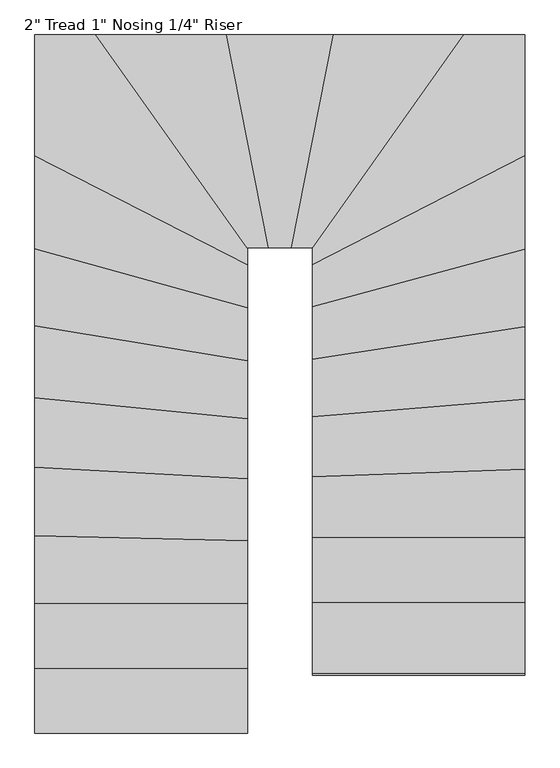
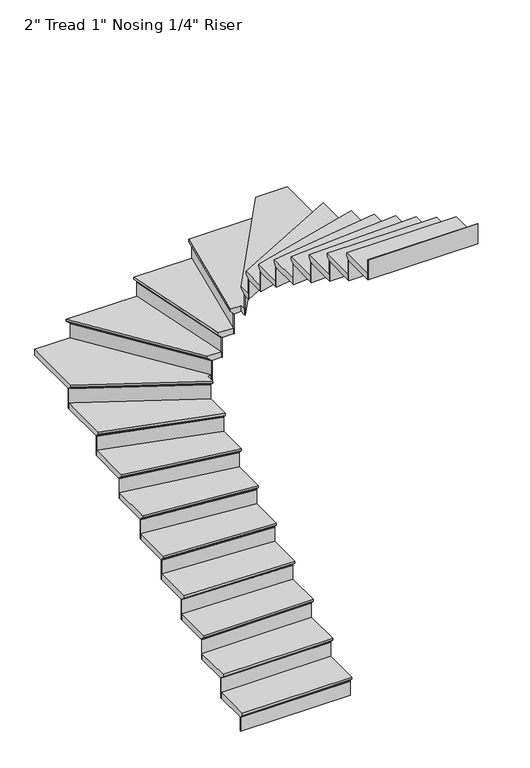
"""IFC4 building model written with IfcOpenShell, lengths in millimetres: stair flight geometry."""

from ifc_helpers import new_model, si_unit, origin, place, context, project, spatial, faceted_brep, source, transform, mapped, element, save


def stair_flight_b5c60846(model_context):
    return source(origin(), model_context, "Body", "Brep", [
        faceted_brep([(-4558.1931367, 3267.4797066, 155.1214286), (-4558.1931367, 3267.4797066, 174.1714286), (-5472.5931367, 3267.4797066, 174.1714286), (-5472.5931367, 3267.4797066, 155.1214286), (-4558.1931367, 3292.8797066, 129.7214286), (-5472.5931367, 3292.8797066, 129.7214286), (-4558.1931367, 3572.2797066, 174.1714286), (-5472.5931367, 3572.2797066, 174.1714286), (-5472.5931367, 3292.8797066, 123.3714286), (-5472.5931367, 3572.2797066, 123.3714286), (-4558.1931367, 3572.2797066, 123.3714286), (-4558.1931367, 3292.8797066, 123.3714286)], [[[0, 1, 2, 3]], [[4, 0, 3, 5]], [[2, 1, 6, 7]], [[8, 9, 10, 11]], [[2, 7, 9, 8, 5, 3]], [[8, 11, 4, 5]], [[6, 1, 0, 4, 11, 10]], [[7, 6, 10, 9]]]),
        faceted_brep([(-4558.1931367, 3292.8797066, 123.3714286), (-4558.1931367, 3292.8797066, 0.0), (-4558.1931367, 3299.2297066, 0.0), (-4558.1931367, 3299.2297066, 123.3714286), (-5472.5931367, 3292.8797066, 123.3714286), (-5472.5931367, 3299.2297066, 123.3714286), (-5472.5931367, 3299.2297066, 0.0), (-5472.5931367, 3292.8797066, 0.0)], [[[0, 1, 2, 3]], [[4, 5, 6, 7]], [[1, 0, 4, 7]], [[2, 1, 7, 6]], [[3, 2, 6, 5]], [[0, 3, 5, 4]]]),
        faceted_brep([(-4558.1931367, 3572.2797066, 297.5428571), (-4558.1931367, 3572.2797066, 123.3714286), (-4558.1931367, 3578.6297066, 123.3714286), (-4558.1931367, 3578.6297066, 297.5428571), (-5472.5931367, 3572.2797066, 297.5428571), (-5472.5931367, 3578.6297066, 297.5428571), (-5472.5931367, 3578.6297066, 123.3714286), (-5472.5931367, 3572.2797066, 123.3714286)], [[[0, 1, 2, 3]], [[4, 5, 6, 7]], [[1, 0, 4, 7]], [[2, 1, 7, 6]], [[3, 2, 6, 5]], [[0, 3, 5, 4]]]),
        faceted_brep([(-5472.5931367, 3546.8797066, 348.3428571), (-4558.1931367, 3546.8797066, 348.3428571), (-4558.1931367, 3851.6797066, 348.3428571), (-5472.5931367, 3851.6797066, 348.3428571), (-5472.5931367, 3572.2797066, 297.5428571), (-5472.5931367, 3851.6797066, 297.5428571), (-4558.1931367, 3851.6797066, 297.5428571), (-4558.1931367, 3572.2797066, 297.5428571), (-5472.5931367, 3572.2797066, 303.8928571), (-5472.5931367, 3546.8797066, 329.2928571), (-4558.1931367, 3572.2797066, 303.8928571), (-4558.1931367, 3546.8797066, 329.2928571)], [[[0, 1, 2, 3]], [[4, 5, 6, 7]], [[0, 3, 5, 4, 8, 9]], [[4, 7, 10, 8]], [[2, 1, 11, 10, 7, 6]], [[3, 2, 6, 5]], [[11, 1, 0, 9]], [[10, 11, 9, 8]]]),
        faceted_brep([(-4558.1931367, 3851.6797066, 471.7142857), (-4558.1931367, 3851.6797066, 297.5428571), (-4558.1931367, 3858.0297066, 297.5428571), (-4558.1931367, 3858.0297066, 471.7142857), (-5472.5931367, 3851.6797066, 471.7142857), (-5472.5931367, 3858.0297066, 471.7142857), (-5472.5931367, 3858.0297066, 297.5428571), (-5472.5931367, 3851.6797066, 297.5428571)], [[[0, 1, 2, 3]], [[4, 5, 6, 7]], [[1, 0, 4, 7]], [[2, 1, 7, 6]], [[3, 2, 6, 5]], [[0, 3, 5, 4]]]),
        faceted_brep([(-5472.5931367, 3826.2797066, 522.5142857), (-4558.1931367, 3826.2797066, 522.5142857), (-4558.1931367, 4120.4786565, 522.5142857), (-5472.5931367, 4141.6944283, 522.5142857), (-5472.5931367, 3851.6797066, 471.7142857), (-5472.5931367, 4141.6944283, 471.7142857), (-4558.1931367, 4120.4786565, 471.7142857), (-4558.1931367, 3851.6797066, 471.7142857), (-5472.5931367, 3851.6797066, 478.0642857), (-5472.5931367, 3826.2797066, 503.4642857), (-4558.1931367, 3851.6797066, 478.0642857), (-4558.1931367, 3826.2797066, 503.4642857)], [[[0, 1, 2, 3]], [[4, 5, 6, 7]], [[0, 3, 5, 4, 8, 9]], [[4, 7, 10, 8]], [[2, 1, 11, 10, 7, 6]], [[3, 2, 6, 5]], [[11, 1, 0, 9]], [[10, 11, 9, 8]]]),
        faceted_brep([(-4558.1931367, 4120.4786565, 645.8857143), (-4558.1931367, 4120.4786565, 471.7142857), (-4558.1931367, 4126.8303655, 471.7142857), (-4558.1931367, 4126.8303655, 645.8857143), (-5472.5931367, 4141.6944283, 645.8857143), (-5472.5931367, 4148.0461372, 645.8857143), (-5472.5931367, 4148.0461372, 471.7142857), (-5472.5931367, 4141.6944283, 471.7142857)], [[[0, 1, 2, 3]], [[4, 5, 6, 7]], [[1, 0, 4, 7]], [[2, 1, 7, 6]], [[3, 2, 6, 5]], [[0, 3, 5, 4]]]),
        faceted_brep([(-5472.5931367, 4116.2875924, 696.6857143), (-4558.1931367, 4095.0718207, 696.6857143), (-4558.1931367, 4385.6939265, 696.6857143), (-5472.5931367, 4435.3403065, 696.6857143), (-5472.5931367, 4141.6944283, 645.8857143), (-5472.5931367, 4435.3403065, 645.8857143), (-4558.1931367, 4385.6939265, 645.8857143), (-4558.1931367, 4120.4786565, 645.8857143), (-5472.5931367, 4141.6944283, 652.2357143), (-5472.5931367, 4116.2875924, 677.6357143), (-4558.1931367, 4120.4786565, 652.2357143), (-4558.1931367, 4095.0718207, 677.6357143)], [[[0, 1, 2, 3]], [[4, 5, 6, 7]], [[0, 3, 5, 4, 8, 9]], [[4, 7, 10, 8]], [[2, 1, 11, 10, 7, 6]], [[3, 2, 6, 5]], [[11, 1, 0, 9]], [[10, 11, 9, 8]]]),
        faceted_brep([(-4558.1931367, 4385.6939265, 820.0571429), (-4558.1931367, 4385.6939265, 645.8857143), (-4558.1931367, 4392.053279, 645.8857143), (-4558.1931367, 4392.053279, 820.0571429), (-5472.5931367, 4435.3403065, 820.0571429), (-5472.5931367, 4441.699659, 820.0571429), (-5472.5931367, 4441.699659, 645.8857143), (-5472.5931367, 4435.3403065, 645.8857143)], [[[0, 1, 2, 3]], [[4, 5, 6, 7]], [[1, 0, 4, 7]], [[2, 1, 7, 6]], [[3, 2, 6, 5]], [[0, 3, 5, 4]]]),
        faceted_brep([(-5472.5931367, 4409.9028966, 870.8571429), (-4558.1931367, 4360.2565166, 870.8571429), (-4558.1931367, 4645.138633, 870.8571429), (-5472.5931367, 4734.864762, 870.8571429), (-5472.5931367, 4435.3403065, 820.0571429), (-5472.5931367, 4734.864762, 820.0571429), (-4558.1931367, 4645.138633, 820.0571429), (-4558.1931367, 4385.6939265, 820.0571429), (-5472.5931367, 4435.3403065, 826.4071429), (-5472.5931367, 4409.9028966, 851.8071429), (-4558.1931367, 4385.6939265, 826.4071429), (-4558.1931367, 4360.2565166, 851.8071429)], [[[0, 1, 2, 3]], [[4, 5, 6, 7]], [[0, 3, 5, 4, 8, 9]], [[4, 7, 10, 8]], [[2, 1, 11, 10, 7, 6]], [[3, 2, 6, 5]], [[11, 1, 0, 9]], [[10, 11, 9, 8]]]),
        faceted_brep([(-4558.1931367, 4645.138633, 994.2285714), (-4558.1931367, 4645.138633, 820.0571429), (-4558.1931367, 4651.5191307, 820.0571429), (-4558.1931367, 4651.5191307, 994.2285714), (-5472.5931367, 4734.864762, 994.2285714), (-5472.5931367, 4741.2452597, 994.2285714), (-5472.5931367, 4741.2452597, 820.0571429), (-5472.5931367, 4734.864762, 820.0571429)], [[[0, 1, 2, 3]], [[4, 5, 6, 7]], [[1, 0, 4, 7]], [[2, 1, 7, 6]], [[3, 2, 6, 5]], [[0, 3, 5, 4]]]),
        faceted_brep([(-5472.5931367, 4709.3427711, 1045.0285714), (-4558.1931367, 4619.6166421, 1045.0285714), (-4558.1931367, 4894.3915533, 1045.0285714), (-5472.5931367, 5044.8509686, 1045.0285714), (-5472.5931367, 4734.864762, 994.2285714), (-5472.5931367, 5044.8509686, 994.2285714), (-4558.1931367, 4894.3915533, 994.2285714), (-4558.1931367, 4645.138633, 994.2285714), (-5472.5931367, 4734.864762, 1000.5785714), (-5472.5931367, 4709.3427711, 1025.9785714), (-4558.1931367, 4645.138633, 1000.5785714), (-4558.1931367, 4619.6166421, 1025.9785714)], [[[0, 1, 2, 3]], [[4, 5, 6, 7]], [[0, 3, 5, 4, 8, 9]], [[4, 7, 10, 8]], [[2, 1, 11, 10, 7, 6]], [[3, 2, 6, 5]], [[11, 1, 0, 9]], [[10, 11, 9, 8]]]),
        faceted_brep([(-4558.1931367, 4894.3915533, 1168.4), (-4558.1931367, 4894.3915533, 994.2285714), (-4558.1931367, 4900.8269419, 994.2285714), (-4558.1931367, 4900.8269419, 1168.4), (-5472.5931367, 5044.8509686, 1168.4), (-5472.5931367, 5051.2863571, 1168.4), (-5472.5931367, 5051.2863571, 994.2285714), (-5472.5931367, 5044.8509686, 994.2285714)], [[[0, 1, 2, 3]], [[4, 5, 6, 7]], [[1, 0, 4, 7]], [[2, 1, 7, 6]], [[3, 2, 6, 5]], [[0, 3, 5, 4]]]),
        faceted_brep([(-5472.5931367, 5019.1094142, 1219.2), (-4558.1931367, 4868.6499989, 1219.2), (-4558.1931367, 5122.9607516, 1219.2), (-5472.5931367, 5376.3124961, 1219.2), (-5472.5931367, 5044.8509686, 1168.4), (-5472.5931367, 5376.3124961, 1168.4), (-4558.1931367, 5122.9607516, 1168.4), (-4558.1931367, 4894.3915533, 1168.4), (-5472.5931367, 5044.8509686, 1174.75), (-5472.5931367, 5019.1094142, 1200.15), (-4558.1931367, 4894.3915533, 1174.75), (-4558.1931367, 4868.6499989, 1200.15)], [[[0, 1, 2, 3]], [[4, 5, 6, 7]], [[0, 3, 5, 4, 8, 9]], [[4, 7, 10, 8]], [[2, 1, 11, 10, 7, 6]], [[3, 2, 6, 5]], [[11, 1, 0, 9]], [[10, 11, 9, 8]]]),
        faceted_brep([(-4558.1931367, 5122.9607516, 1342.5714286), (-4558.1931367, 5122.9607516, 1168.4), (-4558.1931367, 5129.5499809, 1168.4), (-4558.1931367, 5129.5499809, 1342.5714286), (-5472.5931367, 5376.3124961, 1342.5714286), (-5472.5931367, 5382.9017254, 1342.5714286), (-5472.5931367, 5382.9017254, 1168.4), (-5472.5931367, 5376.3124961, 1168.4)], [[[0, 1, 2, 3]], [[4, 5, 6, 7]], [[1, 0, 4, 7]], [[2, 1, 7, 6]], [[3, 2, 6, 5]], [[0, 3, 5, 4]]]),
        faceted_brep([(-5472.5931367, 5349.9555788, 1393.3714286), (-4558.1931367, 5096.6038343, 1393.3714286), (-4558.1931367, 5308.2874264, 1393.3714286), (-5472.5931367, 5777.1120477, 1393.3714286), (-5472.5931367, 5376.3124961, 1342.5714286), (-5472.5931367, 5777.1120477, 1342.5714286), (-4558.1931367, 5308.2874264, 1342.5714286), (-4558.1931367, 5122.9607516, 1342.5714286), (-5472.5931367, 5376.3124961, 1348.9214286), (-5472.5931367, 5349.9555788, 1374.3214286), (-4558.1931367, 5122.9607516, 1348.9214286), (-4558.1931367, 5096.6038343, 1374.3214286)], [[[0, 1, 2, 3]], [[4, 5, 6, 7]], [[0, 3, 5, 4, 8, 9]], [[4, 7, 10, 8]], [[2, 1, 11, 10, 7, 6]], [[3, 2, 6, 5]], [[11, 1, 0, 9]], [[10, 11, 9, 8]]]),
        faceted_brep([(-4558.1931367, 5308.2874264, 1516.7428571), (-4558.1931367, 5308.2874264, 1342.5714286), (-4558.1931367, 5315.4234096, 1342.5714286), (-4558.1931367, 5315.4234096, 1516.7428571), (-5472.5931367, 5777.1120477, 1516.7428571), (-5472.5931367, 5784.2480309, 1516.7428571), (-5472.5931367, 5784.2480309, 1342.5714286), (-5472.5931367, 5777.1120477, 1342.5714286)], [[[0, 1, 2, 3]], [[4, 5, 6, 7]], [[1, 0, 4, 7]], [[2, 1, 7, 6]], [[3, 2, 6, 5]], [[0, 3, 5, 4]]]),
        faceted_brep([(-5178.912003, 6268.4113984, 1567.5428571), (-5472.5931367, 6268.4113984, 1567.5428571), (-5472.5931367, 5748.5681152, 1567.5428571), (-4558.1931367, 5279.7434939, 1567.5428571), (-4558.1931367, 5354.0113984, 1567.5428571), (-4528.6380538, 5354.0113984, 1567.5428571), (-5472.5931367, 6268.4113984, 1516.7428571), (-5178.912003, 6268.4113984, 1516.7428571), (-4528.6380538, 5354.0113984, 1516.7428571), (-4558.1931367, 5354.0113984, 1516.7428571), (-4558.1931367, 5308.2874264, 1516.7428571), (-5472.5931367, 5777.1120477, 1516.7428571), (-5472.5931367, 5777.1120477, 1523.0928571), (-5472.5931367, 5748.5681152, 1548.4928571), (-4558.1931367, 5308.2874264, 1523.0928571), (-4558.1931367, 5279.7434939, 1548.4928571)], [[[0, 1, 2, 3, 4, 5]], [[6, 7, 8, 9, 10, 11]], [[1, 0, 7, 6]], [[2, 1, 6, 11, 12, 13]], [[11, 10, 14, 12]], [[4, 3, 15, 14, 10, 9]], [[5, 4, 9, 8]], [[0, 5, 8, 7]], [[15, 3, 2, 13]], [[14, 15, 13, 12]]]),
        faceted_brep([(-4528.6380538, 5354.0113984, 1690.9142857), (-4528.6380538, 5354.0113984, 1516.7428571), (-4520.846079, 5354.0113984, 1516.7428571), (-4520.846079, 5354.0113984, 1690.9142857), (-5178.912003, 6268.4113984, 1690.9142857), (-5171.1200282, 6268.4113984, 1690.9142857), (-5171.1200282, 6268.4113984, 1516.7428571), (-5178.912003, 6268.4113984, 1516.7428571)], [[[0, 1, 2, 3]], [[4, 5, 6, 7]], [[1, 0, 4, 7]], [[2, 1, 7, 6]], [[3, 2, 6, 5]], [[0, 3, 5, 4]]]),
        faceted_brep([(-5210.0799021, 6268.4113984, 1741.7142857), (-4559.805953, 5354.0113984, 1741.7142857), (-4442.1839667, 5354.0113984, 1741.7142857), (-4622.4248231, 6268.4113984, 1741.7142857), (-5178.912003, 6268.4113984, 1690.9142857), (-4622.4248231, 6268.4113984, 1690.9142857), (-4442.1839667, 5354.0113984, 1690.9142857), (-4528.6380538, 5354.0113984, 1690.9142857), (-5178.912003, 6268.4113984, 1697.2642857), (-5210.0799021, 6268.4113984, 1722.6642857), (-4528.6380538, 5354.0113984, 1697.2642857), (-4559.805953, 5354.0113984, 1722.6642857)], [[[0, 1, 2, 3]], [[4, 5, 6, 7]], [[0, 3, 5, 4, 8, 9]], [[4, 7, 10, 8]], [[2, 1, 11, 10, 7, 6]], [[3, 2, 6, 5]], [[11, 1, 0, 9]], [[10, 11, 9, 8]]]),
        faceted_brep([(-4442.1839667, 5354.0113984, 1865.0857143), (-4442.1839667, 5354.0113984, 1690.9142857), (-4435.7117813, 5354.0113984, 1690.9142857), (-4435.7117813, 5354.0113984, 1865.0857143), (-4622.4248231, 6268.4113984, 1865.0857143), (-4615.9526376, 6268.4113984, 1865.0857143), (-4615.9526376, 6268.4113984, 1690.9142857), (-4622.4248231, 6268.4113984, 1690.9142857)], [[[0, 1, 2, 3]], [[4, 5, 6, 7]], [[1, 0, 4, 7]], [[2, 1, 7, 6]], [[3, 2, 6, 5]], [[0, 3, 5, 4]]]),
        faceted_brep([(-4648.3135648, 6268.4113984, 1915.8857143), (-4468.0727085, 5354.0113984, 1915.8857143), (-4343.0248231, 5354.0113984, 1915.8857143), (-4162.7839667, 6268.4113984, 1915.8857143), (-4622.4248231, 6268.4113984, 1865.0857143), (-4162.7839667, 6268.4113984, 1865.0857143), (-4343.0248231, 5354.0113984, 1865.0857143), (-4442.1839667, 5354.0113984, 1865.0857143), (-4622.4248231, 6268.4113984, 1871.4357143), (-4648.3135648, 6268.4113984, 1896.8357143), (-4442.1839667, 5354.0113984, 1871.4357143), (-4468.0727085, 5354.0113984, 1896.8357143)], [[[0, 1, 2, 3]], [[4, 5, 6, 7]], [[0, 3, 5, 4, 8, 9]], [[4, 7, 10, 8]], [[2, 1, 11, 10, 7, 6]], [[3, 2, 6, 5]], [[11, 1, 0, 9]], [[10, 11, 9, 8]]]),
        faceted_brep([(-4343.0248231, 5354.0113984, 2039.2571429), (-4343.0248231, 5354.0113984, 1865.0857143), (-4336.5526376, 5354.0113984, 1865.0857143), (-4336.5526376, 5354.0113984, 2039.2571429), (-4162.7839667, 6268.4113984, 2039.2571429), (-4156.3117813, 6268.4113984, 2039.2571429), (-4156.3117813, 6268.4113984, 1865.0857143), (-4162.7839667, 6268.4113984, 1865.0857143)], [[[0, 1, 2, 3]], [[4, 5, 6, 7]], [[1, 0, 4, 7]], [[2, 1, 7, 6]], [[3, 2, 6, 5]], [[0, 3, 5, 4]]]),
        faceted_brep([(-4188.6727085, 6268.4113984, 2090.0571429), (-4368.9135648, 5354.0113984, 2090.0571429), (-4278.7931367, 5354.0113984, 2090.0571429), (-4278.7931367, 5307.9159239, 2090.0571429), (-3595.738472, 6268.4113984, 2090.0571429), (-4162.7839667, 6268.4113984, 2039.2571429), (-3595.738472, 6268.4113984, 2039.2571429), (-4278.7931367, 5307.9159239, 2039.2571429), (-4278.7931367, 5354.0113984, 2039.2571429), (-4343.0248231, 5354.0113984, 2039.2571429), (-4162.7839667, 6268.4113984, 2045.6071429), (-4188.6727085, 6268.4113984, 2071.0071429), (-4343.0248231, 5354.0113984, 2045.6071429), (-4368.9135648, 5354.0113984, 2071.0071429)], [[[0, 1, 2, 3, 4]], [[5, 6, 7, 8, 9]], [[0, 4, 6, 5, 10, 11]], [[5, 9, 12, 10]], [[2, 1, 13, 12, 9, 8]], [[3, 2, 8, 7]], [[4, 3, 7, 6]], [[13, 1, 0, 11]], [[12, 13, 11, 10]]]),
        faceted_brep([(-4278.7931367, 5307.9159239, 2213.4285714), (-4278.7931367, 5307.9159239, 2039.2571429), (-4278.7931367, 5296.9590314, 2039.2571429), (-4278.7931367, 5296.9590314, 2213.4285714), (-3595.738472, 6268.4113984, 2213.4285714), (-3587.9464972, 6268.4113984, 2213.4285714), (-3587.9464972, 6268.4113984, 2039.2571429), (-3595.738472, 6268.4113984, 2039.2571429)], [[[0, 1, 2, 3]], [[4, 5, 6, 7]], [[1, 0, 4, 7]], [[2, 1, 7, 6]], [[3, 2, 6, 5]], [[0, 3, 5, 4]]]),
        faceted_brep([(-3364.3931367, 5720.0241827, 2264.2285714), (-3364.3931367, 6268.4113984, 2264.2285714), (-3626.9063712, 6268.4113984, 2264.2285714), (-4278.7931367, 5351.7434939, 2264.2285714), (-4278.7931367, 5251.1995614, 2264.2285714), (-3364.3931367, 6268.4113984, 2213.4285714), (-3364.3931367, 5720.0241827, 2213.4285714), (-4278.7931367, 5251.1995614, 2213.4285714), (-4278.7931367, 5307.9159239, 2213.4285714), (-3595.738472, 6268.4113984, 2213.4285714), (-3595.738472, 6268.4113984, 2219.7785714), (-3626.9063712, 6268.4113984, 2245.1785714), (-4278.7931367, 5307.9159239, 2219.7785714), (-4278.7931367, 5351.7434939, 2245.1785714)], [[[0, 1, 2, 3, 4]], [[5, 6, 7, 8, 9]], [[1, 0, 6, 5]], [[2, 1, 5, 9, 10, 11]], [[9, 8, 12, 10]], [[4, 3, 13, 12, 8, 7]], [[0, 4, 7, 6]], [[13, 3, 2, 11]], [[12, 13, 11, 10]]]),
        faceted_brep([(-4278.7931367, 5251.1995614, 2387.6), (-4278.7931367, 5251.1995614, 2213.4285714), (-4278.7931367, 5244.0635782, 2213.4285714), (-4278.7931367, 5244.0635782, 2387.6), (-3364.3931367, 5720.0241827, 2387.6), (-3364.3931367, 5712.8881995, 2387.6), (-3364.3931367, 5712.8881995, 2213.4285714), (-3364.3931367, 5720.0241827, 2213.4285714)], [[[0, 1, 2, 3]], [[4, 5, 6, 7]], [[1, 0, 4, 7]], [[2, 1, 7, 6]], [[3, 2, 6, 5]], [[0, 3, 5, 4]]]),
        faceted_brep([(-3364.3931367, 5748.5681152, 2438.4), (-4278.7931367, 5279.7434939, 2438.4), (-4278.7931367, 5073.8765796, 2438.4), (-3364.3931367, 5320.0737347, 2438.4), (-3364.3931367, 5720.0241827, 2387.6), (-3364.3931367, 5320.0737347, 2387.6), (-4278.7931367, 5073.8765796, 2387.6), (-4278.7931367, 5251.1995614, 2387.6), (-3364.3931367, 5720.0241827, 2393.95), (-3364.3931367, 5748.5681152, 2419.35), (-4278.7931367, 5251.1995614, 2393.95), (-4278.7931367, 5279.7434939, 2419.35)], [[[0, 1, 2, 3]], [[4, 5, 6, 7]], [[0, 3, 5, 4, 8, 9]], [[4, 7, 10, 8]], [[2, 1, 11, 10, 7, 6]], [[3, 2, 6, 5]], [[11, 1, 0, 9]], [[10, 11, 9, 8]]]),
        faceted_brep([(-4278.7931367, 5073.8765796, 2561.7714286), (-4278.7931367, 5073.8765796, 2387.6), (-4278.7931367, 5067.3004423, 2387.6), (-4278.7931367, 5067.3004423, 2561.7714286), (-3364.3931367, 5320.0737347, 2561.7714286), (-3364.3931367, 5313.4975973, 2561.7714286), (-3364.3931367, 5313.4975973, 2387.6), (-3364.3931367, 5320.0737347, 2387.6)], [[[0, 1, 2, 3]], [[4, 5, 6, 7]], [[1, 0, 4, 7]], [[2, 1, 7, 6]], [[3, 2, 6, 5]], [[0, 3, 5, 4]]]),
        faceted_brep([(-3364.3931367, 5346.3782841, 2612.5714286), (-4278.7931367, 5100.1811291, 2612.5714286), (-4278.7931367, 4849.2003072, 2612.5714286), (-3364.3931367, 4987.183977, 2612.5714286), (-3364.3931367, 5320.0737347, 2561.7714286), (-3364.3931367, 4987.183977, 2561.7714286), (-4278.7931367, 4849.2003072, 2561.7714286), (-4278.7931367, 5073.8765796, 2561.7714286), (-3364.3931367, 5320.0737347, 2568.1214286), (-3364.3931367, 5346.3782841, 2593.5214286), (-4278.7931367, 5073.8765796, 2568.1214286), (-4278.7931367, 5100.1811291, 2593.5214286)], [[[0, 1, 2, 3]], [[4, 5, 6, 7]], [[0, 3, 5, 4, 8, 9]], [[4, 7, 10, 8]], [[2, 1, 11, 10, 7, 6]], [[3, 2, 6, 5]], [[11, 1, 0, 9]], [[10, 11, 9, 8]]]),
        faceted_brep([(-4278.7931367, 4849.2003072, 2735.9428571), (-4278.7931367, 4849.2003072, 2561.7714286), (-4278.7931367, 4842.7784161, 2561.7714286), (-4278.7931367, 4842.7784161, 2735.9428571), (-3364.3931367, 4987.183977, 2735.9428571), (-3364.3931367, 4980.7620859, 2735.9428571), (-3364.3931367, 4980.7620859, 2561.7714286), (-3364.3931367, 4987.183977, 2561.7714286)], [[[0, 1, 2, 3]], [[4, 5, 6, 7]], [[1, 0, 4, 7]], [[2, 1, 7, 6]], [[3, 2, 6, 5]], [[0, 3, 5, 4]]]),
        faceted_brep([(-3364.3931367, 5012.8715415, 2786.7428571), (-4278.7931367, 4874.8878717, 2786.7428571), (-4278.7931367, 4602.2821821, 2786.7428571), (-3364.3931367, 4675.7136896, 2786.7428571), (-3364.3931367, 4987.183977, 2735.9428571), (-3364.3931367, 4675.7136896, 2735.9428571), (-4278.7931367, 4602.2821821, 2735.9428571), (-4278.7931367, 4849.2003072, 2735.9428571), (-3364.3931367, 4987.183977, 2742.2928571), (-3364.3931367, 5012.8715415, 2767.6928571), (-4278.7931367, 4849.2003072, 2742.2928571), (-4278.7931367, 4874.8878717, 2767.6928571)], [[[0, 1, 2, 3]], [[4, 5, 6, 7]], [[0, 3, 5, 4, 8, 9]], [[4, 7, 10, 8]], [[2, 1, 11, 10, 7, 6]], [[3, 2, 6, 5]], [[11, 1, 0, 9]], [[10, 11, 9, 8]]]),
        faceted_brep([(-4278.7931367, 4602.2821821, 2910.1142857), (-4278.7931367, 4602.2821821, 2735.9428571), (-4278.7931367, 4595.9117395, 2735.9428571), (-4278.7931367, 4595.9117395, 2910.1142857), (-3364.3931367, 4675.7136896, 2910.1142857), (-3364.3931367, 4669.343247, 2910.1142857), (-3364.3931367, 4669.343247, 2735.9428571), (-3364.3931367, 4675.7136896, 2735.9428571)], [[[0, 1, 2, 3]], [[4, 5, 6, 7]], [[1, 0, 4, 7]], [[2, 1, 7, 6]], [[3, 2, 6, 5]], [[0, 3, 5, 4]]]),
        faceted_brep([(-3364.3931367, 4701.1954603, 2960.9142857), (-4278.7931367, 4627.7639528, 2960.9142857), (-4278.7931367, 4344.3894136, 2960.9142857), (-3364.3931367, 4374.9416513, 2960.9142857), (-3364.3931367, 4675.7136896, 2910.1142857), (-3364.3931367, 4374.9416513, 2910.1142857), (-4278.7931367, 4344.3894136, 2910.1142857), (-4278.7931367, 4602.2821821, 2910.1142857), (-3364.3931367, 4675.7136896, 2916.4642857), (-3364.3931367, 4701.1954603, 2941.8642857), (-4278.7931367, 4602.2821821, 2916.4642857), (-4278.7931367, 4627.7639528, 2941.8642857)], [[[0, 1, 2, 3]], [[4, 5, 6, 7]], [[0, 3, 5, 4, 8, 9]], [[4, 7, 10, 8]], [[2, 1, 11, 10, 7, 6]], [[3, 2, 6, 5]], [[11, 1, 0, 9]], [[10, 11, 9, 8]]]),
        faceted_brep([(-4278.7931367, 4344.3894136, 3084.2857143), (-4278.7931367, 4344.3894136, 2910.1142857), (-4278.7931367, 4338.0358701, 2910.1142857), (-4278.7931367, 4338.0358701, 3084.2857143), (-3364.3931367, 4374.9416513, 3084.2857143), (-3364.3931367, 4368.5881078, 3084.2857143), (-3364.3931367, 4368.5881078, 2910.1142857), (-3364.3931367, 4374.9416513, 2910.1142857)], [[[0, 1, 2, 3]], [[4, 5, 6, 7]], [[1, 0, 4, 7]], [[2, 1, 7, 6]], [[3, 2, 6, 5]], [[0, 3, 5, 4]]]),
        faceted_brep([(-3364.3931367, 4400.3558254, 3135.0857143), (-4278.7931367, 4369.8035877, 3135.0857143), (-4278.7931367, 4080.2797066, 3135.0857143), (-3364.3931367, 4080.2797066, 3135.0857143), (-3364.3931367, 4374.9416513, 3084.2857143), (-3364.3931367, 4080.2797066, 3084.2857143), (-4278.7931367, 4080.2797066, 3084.2857143), (-4278.7931367, 4344.3894136, 3084.2857143), (-3364.3931367, 4374.9416513, 3090.6357143), (-3364.3931367, 4400.3558254, 3116.0357143), (-4278.7931367, 4344.3894136, 3090.6357143), (-4278.7931367, 4369.8035877, 3116.0357143)], [[[0, 1, 2, 3]], [[4, 5, 6, 7]], [[0, 3, 5, 4, 8, 9]], [[4, 7, 10, 8]], [[2, 1, 11, 10, 7, 6]], [[3, 2, 6, 5]], [[11, 1, 0, 9]], [[10, 11, 9, 8]]]),
        faceted_brep([(-4278.7931367, 4080.2797066, 3258.4571429), (-4278.7931367, 4080.2797066, 3084.2857143), (-4278.7931367, 4073.9297066, 3084.2857143), (-4278.7931367, 4073.9297066, 3258.4571429), (-3364.3931367, 4080.2797066, 3258.4571429), (-3364.3931367, 4073.9297066, 3258.4571429), (-3364.3931367, 4073.9297066, 3084.2857143), (-3364.3931367, 4080.2797066, 3084.2857143)], [[[0, 1, 2, 3]], [[4, 5, 6, 7]], [[1, 0, 4, 7]], [[2, 1, 7, 6]], [[3, 2, 6, 5]], [[0, 3, 5, 4]]]),
        faceted_brep([(-3364.3931367, 4105.6797066, 3309.2571429), (-4278.7931367, 4105.6797066, 3309.2571429), (-4278.7931367, 3800.8797066, 3309.2571429), (-3364.3931367, 3800.8797066, 3309.2571429), (-3364.3931367, 4080.2797066, 3258.4571429), (-3364.3931367, 3800.8797066, 3258.4571429), (-4278.7931367, 3800.8797066, 3258.4571429), (-4278.7931367, 4080.2797066, 3258.4571429), (-3364.3931367, 4080.2797066, 3264.8071429), (-3364.3931367, 4105.6797066, 3290.2071429), (-4278.7931367, 4080.2797066, 3264.8071429), (-4278.7931367, 4105.6797066, 3290.2071429)], [[[0, 1, 2, 3]], [[4, 5, 6, 7]], [[0, 3, 5, 4, 8, 9]], [[4, 7, 10, 8]], [[2, 1, 11, 10, 7, 6]], [[3, 2, 6, 5]], [[11, 1, 0, 9]], [[10, 11, 9, 8]]]),
        faceted_brep([(-4278.7931367, 3800.8797066, 3432.6285714), (-4278.7931367, 3800.8797066, 3258.4571429), (-4278.7931367, 3794.5297066, 3258.4571429), (-4278.7931367, 3794.5297066, 3432.6285714), (-3364.3931367, 3800.8797066, 3432.6285714), (-3364.3931367, 3794.5297066, 3432.6285714), (-3364.3931367, 3794.5297066, 3258.4571429), (-3364.3931367, 3800.8797066, 3258.4571429)], [[[0, 1, 2, 3]], [[4, 5, 6, 7]], [[1, 0, 4, 7]], [[2, 1, 7, 6]], [[3, 2, 6, 5]], [[0, 3, 5, 4]]]),
        faceted_brep([(-4278.7931367, 3521.4797066, 3606.8), (-4278.7931367, 3521.4797066, 3432.6285714), (-4278.7931367, 3515.1297066, 3432.6285714), (-4278.7931367, 3515.1297066, 3606.8), (-3364.3931367, 3521.4797066, 3606.8), (-3364.3931367, 3515.1297066, 3606.8), (-3364.3931367, 3515.1297066, 3432.6285714), (-3364.3931367, 3521.4797066, 3432.6285714)], [[[0, 1, 2, 3]], [[4, 5, 6, 7]], [[1, 0, 4, 7]], [[2, 1, 7, 6]], [[3, 2, 6, 5]], [[0, 3, 5, 4]]]),
        faceted_brep([(-3364.3931367, 3826.2797066, 3483.4285714), (-4278.7931367, 3826.2797066, 3483.4285714), (-4278.7931367, 3521.4797066, 3483.4285714), (-3364.3931367, 3521.4797066, 3483.4285714), (-3364.3931367, 3800.8797066, 3432.6285714), (-3364.3931367, 3521.4797066, 3432.6285714), (-4278.7931367, 3521.4797066, 3432.6285714), (-4278.7931367, 3800.8797066, 3432.6285714), (-3364.3931367, 3800.8797066, 3438.9785714), (-3364.3931367, 3826.2797066, 3464.3785714), (-4278.7931367, 3800.8797066, 3438.9785714), (-4278.7931367, 3826.2797066, 3464.3785714)], [[[0, 1, 2, 3]], [[4, 5, 6, 7]], [[0, 3, 5, 4, 8, 9]], [[4, 7, 10, 8]], [[2, 1, 11, 10, 7, 6]], [[3, 2, 6, 5]], [[11, 1, 0, 9]], [[10, 11, 9, 8]]]),
    ])


if __name__ == "__main__":
    model = new_model("IFC4")
    model_context = context("Model", 3, world=origin())
    ifc_project = project(units=[si_unit("LENGTHUNIT", "METRE", prefix="MILLI")], contexts=[model_context])
    site = spatial("IfcSite", under=ifc_project)
    building = spatial("IfcBuilding", under=site)
    placement = place(None, origin())
    stair_flight_shape = stair_flight_b5c60846(model_context)
    element("IfcStairFlight", 1, ObjectType="2\" Tread 1\" Nosing 1/4\" Riser", at=placement, inside=building, context=model_context, shape_type="MappedRepresentation", body=[
        mapped(stair_flight_shape, transform((0.0, 0.0, 0.0), x_axis=(1.0, 0.0, 0.0), y_axis=(0.0, 1.0, 0.0), z_axis=(0.0, 0.0, 1.0))),
    ])
    save(model, "model.ifc")
